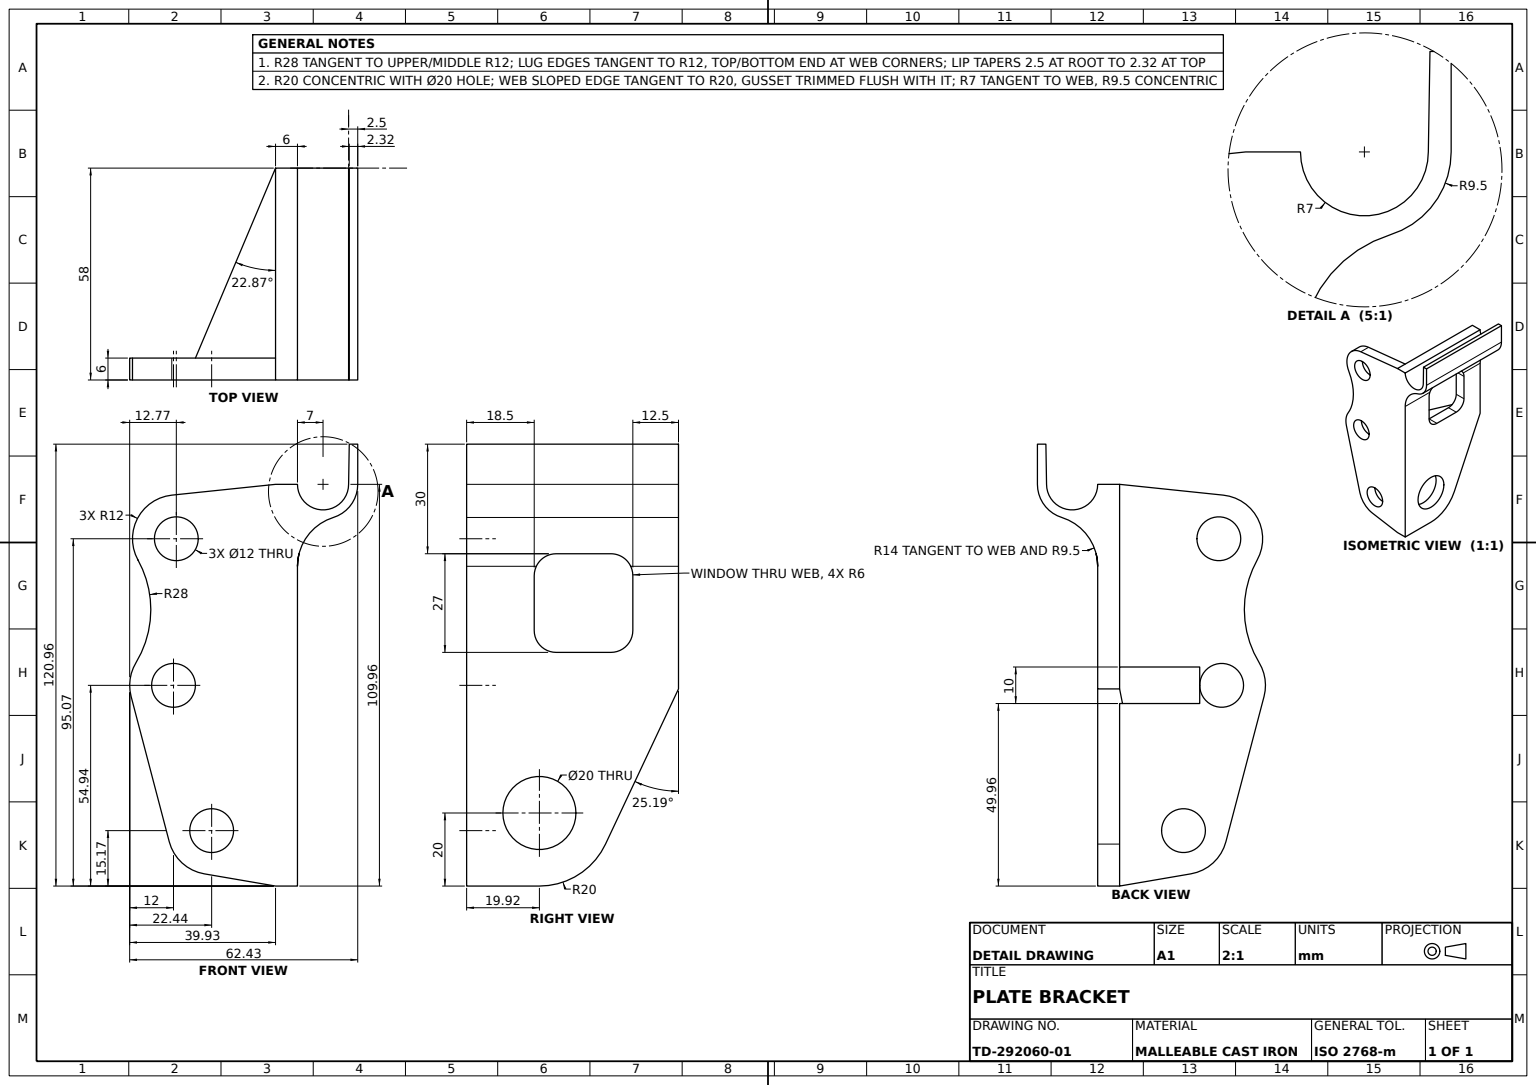
from build123d import *

# Parameters (mm, degrees)
BASE_PLATE_SKETCH_W      = 58
BASE_PLATE_SKETCH_H      = 56
BASE_PLATE_DEPTH         = 6
CHANNEL_WALL_DEPTH       = 58
CHANNEL_GROOVE_CUT_DEPTH = 58
GROOVE_LIP_DEPTH         = 58
SIDE_ARM_DEPTH           = 6
LUG_PLATE_DEPTH          = 6
UPPER_HOLE_SKETCH_R      = 6
UPPER_HOLE_DEPTH         = 6
MIDDLE_HOLE_SKETCH_R     = 10
MIDDLE_HOLE_DEPTH        = 6
GUSSET_DEPTH             = 60
GUSSET_TRIM_CUT_A_DEPTH  = 50
GUSSET_TRIM_CUT_B_DEPTH  = 50
ARM_PROFILE_CUT_DEPTH    = 6
LOWER_HOLE_DEPTH         = 6


with BuildPart() as part:
    # Base Plate Sketch → Base Plate (new body)
    with BuildSketch(Plane.XY):
        with Locations((29, -28)):
            Rectangle(BASE_PLATE_SKETCH_W, BASE_PLATE_SKETCH_H)
    extrude(amount=BASE_PLATE_DEPTH)

    # Channel Wall Sketch → Channel Wall (add)
    with BuildSketch(Plane.ZY):
        with BuildLine():
            Line((0, 0), (-7, 0))
            Line((-7, 0), (-16.5, 0))
            ThreePointArc((-16.5, 0), (-14.652874582, -5.628810766), (-9.829787234, -9.068754281))
            ThreePointArc((-9.829787234, -9.068754281), (-2.722079564, -14.138144724), (0, -22.433234274))
            Line((0, -22.433234274), (0, 0))
        make_face()
    extrude(amount=-CHANNEL_WALL_DEPTH)

    # Channel Groove Sketch → Channel Groove Cut (cut)
    with BuildSketch(Plane.ZY):
        with BuildLine():
            Line((-14, 0), (0, 0))
            ThreePointArc((0, 0), (-7, -7), (-14, 0))
        make_face()
    extrude(amount=-CHANNEL_GROOVE_CUT_DEPTH, mode=Mode.SUBTRACT)

    # Groove Lip Sketch → Groove Lip (add)
    with BuildSketch(Plane.ZY):
        Polygon((-16.5, 0), (-16.5, 11), (-14.179240466, 11), (-14, 0), align=None)
    extrude(amount=-GROOVE_LIP_DEPTH)

    # Side Arm Sketch → Side Arm (add)
    with BuildSketch(Plane.XY.offset(6)):
        with BuildLine():
            Line((58, -109.964049753), (58, -56))
            Line((58, -56), (0, -56))
            Line((0, -56), (19.97833348, -98.476319664))
            ThreePointArc((19.97833348, -98.476319664), (27.35835162, -106.849626412), (38.076434513, -109.964049753))
            Line((38.076434513, -109.964049753), (58, -109.964049753))
        make_face()
    extrude(amount=-SIDE_ARM_DEPTH)

    # Lug Plate Sketch → Lug Plate (add)
    with BuildSketch(Plane(origin=(58, 0, 0), x_dir=(0, 0, -1), z_dir=(1, 0, 0))):
        with BuildLine():
            Line((-6, -109.964049753), (-25.517753411, -106.618685655))
            ThreePointArc((-25.517753411, -106.618685655), (-31.598484509, -103.637669036), (-35.096950284, -97.83917889))
            Line((-35.096950284, -97.83917889), (-45.54096595, -58.069710813))
            ThreePointArc((-45.54096595, -58.069710813), (-45.810409179, -53.300291354), (-44.197856883, -48.803666316))
            ThreePointArc((-44.197856883, -48.803666316), (-40.150792049, -34.831779802), (-43.659207606, -20.715003724))
            ThreePointArc((-43.659207606, -20.715003724), (-43.807215073, -9.350336516), (-34.408466657, -2.959632707))
            Line((-34.408466657, -2.959632707), (-6, 0))
            Line((-6, 0), (-6, -109.964049753))
        make_face()
    extrude(amount=-LUG_PLATE_DEPTH)

    # Upper Hole Sketch → Upper Hole (cut)
    with BuildSketch(Plane.ZY.offset(-52)):
        with Locations((33.165020152, -14.89503554)):
            Circle(UPPER_HOLE_SKETCH_R)
        with Locations((33.934519119, -55.021696385)):
            Circle(UPPER_HOLE_SKETCH_R)
        with Locations((23.490503453, -94.791164461)):
            Circle(UPPER_HOLE_SKETCH_R)
    extrude(amount=-UPPER_HOLE_DEPTH, mode=Mode.SUBTRACT)

    # Middle Hole Sketch → Middle Hole (cut)
    with BuildSketch(Plane.XY.offset(6)):
        with Locations((38.076434513, -89.964049753)):
            Circle(MIDDLE_HOLE_SKETCH_R)
    extrude(amount=-MIDDLE_HOLE_DEPTH, mode=Mode.SUBTRACT)

    # Gusset Sketch → Gusset (add)
    with BuildSketch(Plane(origin=(0, 0, 0), x_dir=(1, 0, 0), z_dir=(0, 1, 0))):
        Polygon((52, -6), (52, -27.93), (0, -6), align=None)
    extrude(amount=-GUSSET_DEPTH)

    # Gusset Trim Sketch A → Gusset Trim Cut A (cut)
    with BuildSketch(Plane(origin=(0, 0, 0), x_dir=(1, 0, 0), z_dir=(0, 1, 0))):
        Polygon((0, -6), (52, -6), (52, -27.93), align=None)
    extrude(amount=-GUSSET_TRIM_CUT_A_DEPTH, mode=Mode.SUBTRACT)

    # Gusset Trim Sketch B → Gusset Trim Cut B (cut)
    with BuildSketch(Plane(origin=(0, 0, 6), x_dir=(-1, 0, 0), z_dir=(0, 0, -1))):
        Polygon((-1.881362005, -60), (0, -56), (0, -60), align=None)
    extrude(amount=-GUSSET_TRIM_CUT_B_DEPTH, mode=Mode.SUBTRACT)

    # Arm Profile Cut Sketch → Arm Profile Cut (cut)
    with BuildSketch(Plane.XY.offset(6)):
        with BuildLine():
            Line((18.5, -46), (33.5, -46))
            ThreePointArc((33.5, -46), (37.742640687, -44.242640687), (39.5, -40))
            Line((39.5, -40), (39.5, -25))
            ThreePointArc((39.5, -25), (37.742640687, -20.757359313), (33.5, -19))
            Line((33.5, -19), (18.5, -19))
            ThreePointArc((18.5, -19), (14.257359313, -20.757359313), (12.5, -25))
            Line((12.5, -25), (12.5, -40))
            ThreePointArc((12.5, -40), (14.257359313, -44.242640687), (18.5, -46))
        make_face()
    extrude(amount=-ARM_PROFILE_CUT_DEPTH, mode=Mode.SUBTRACT)

    # Lower Hole Sketch → Lower Hole (cut)
    with BuildSketch(Plane.XY):
        with BuildLine():
            Line((13.076743256, -22.433234274), (38.923256744, -22.433234274))
            ThreePointArc((38.923256744, -22.433234274), (36.709315008, -19.930453948), (33.5, -19))
            Line((33.5, -19), (18.5, -19))
            ThreePointArc((18.5, -19), (15.290684992, -19.930453948), (13.076743256, -22.433234274))
        make_face()
    extrude(amount=-LOWER_HOLE_DEPTH, mode=Mode.SUBTRACT)


solid = part.part
